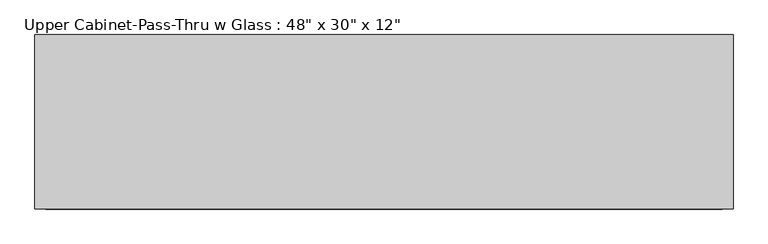
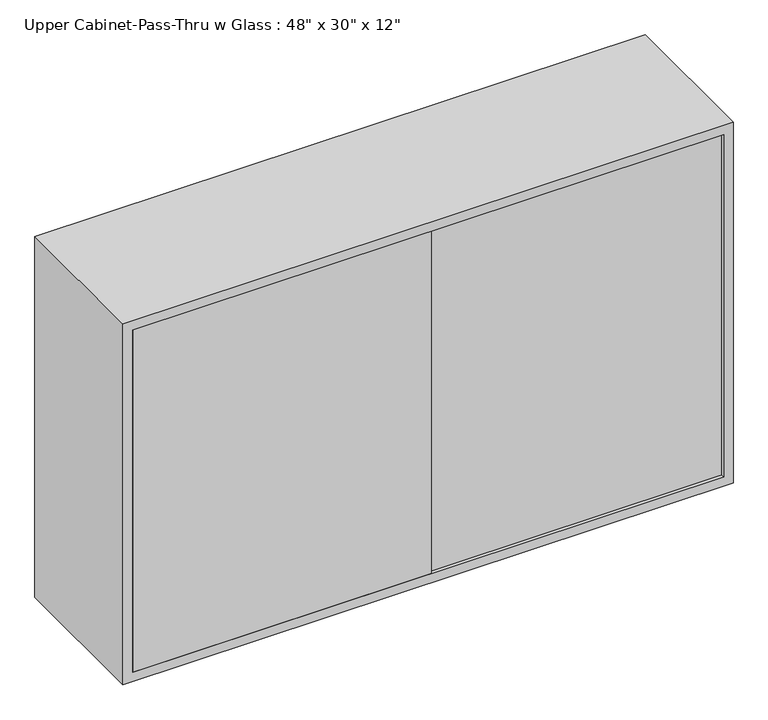
"""IFC4 building model written with IfcOpenShell, lengths in millimetres: furniture geometry."""

from ifc_helpers import new_model, si_unit, frame, origin, place, context, project, spatial, polyline, outline, extrude, source, transform, mapped, element, save


def furniture_f491f192(model_context):
    return source(origin(), model_context, "Body", "SweptSolid", [
        extrude(outline(polyline([(1371.6, 628.3377049), (2133.6, 628.3377049), (2133.6, -590.8622951), (1371.6, -590.8622951), (1371.6, 628.3377049)]), holes=[polyline([(1390.65, 609.2877049), (1390.65, -571.8122951), (2114.55, -571.8122951), (2114.55, 609.2877049), (1390.65, 609.2877049)])]), frame((0.0, -304.8, 0.0), z_axis=(0.0, 1.0, 0.0), x_axis=(0.0, 0.0, 1.0)), (0.0, 0.0, 1.0), 304.8),
        extrude(outline(polyline([(25.0877049, -304.8), (-571.8122951, -304.8), (-571.8122951, -298.45), (25.0877049, -298.45), (25.0877049, -304.8)])), frame((0.0, 0.0, 1390.65), z_axis=(0.0, 0.0, 1.0), x_axis=(1.0, 0.0, 0.0)), (0.0, 0.0, 1.0), 723.9),
        extrude(outline(polyline([(609.2877049, -6.35), (12.3877049, -6.35), (12.3877049, 0.0), (609.2877049, 0.0), (609.2877049, -6.35)])), frame((0.0, 0.0, 1390.65), z_axis=(0.0, 0.0, 1.0), x_axis=(1.0, 0.0, 0.0)), (0.0, 0.0, 1.0), 723.9),
        extrude(outline(polyline([(609.2877049, -298.45), (12.3877049, -298.45), (12.3877049, -292.1), (609.2877049, -292.1), (609.2877049, -298.45)])), frame((0.0, 0.0, 1390.65), z_axis=(0.0, 0.0, 1.0), x_axis=(1.0, 0.0, 0.0)), (0.0, 0.0, 1.0), 723.9),
        extrude(outline(polyline([(25.0877049, -12.7), (-571.8122951, -12.7), (-571.8122951, -6.35), (25.0877049, -6.35), (25.0877049, -12.7)])), frame((0.0, 0.0, 1390.65), z_axis=(0.0, 0.0, 1.0), x_axis=(1.0, 0.0, 0.0)), (0.0, 0.0, 1.0), 723.9),
        extrude(outline(polyline([(609.2877049, -285.75), (-571.8122951, -285.75), (-571.8122951, -19.05), (609.2877049, -19.05), (609.2877049, -285.75)])), frame((0.0, 0.0, 1873.25), z_axis=(0.0, 0.0, 1.0), x_axis=(1.0, 0.0, 0.0)), (0.0, 0.0, 1.0), 12.7),
        extrude(outline(polyline([(609.2877049, -285.75), (-571.8122951, -285.75), (-571.8122951, -19.05), (609.2877049, -19.05), (609.2877049, -285.75)])), frame((0.0, 0.0, 1619.25), z_axis=(0.0, 0.0, 1.0), x_axis=(1.0, 0.0, 0.0)), (0.0, 0.0, 1.0), 12.7),
    ])


if __name__ == "__main__":
    model = new_model("IFC4")
    model_context = context("Model", 3, world=origin())
    ifc_project = project(units=[si_unit("LENGTHUNIT", "METRE", prefix="MILLI")], contexts=[model_context])
    site = spatial("IfcSite", under=ifc_project)
    building = spatial("IfcBuilding", under=site)
    placement = place(None, origin())
    furniture_shape = furniture_f491f192(model_context)
    element("IfcFurniture", 1, ObjectType="Upper Cabinet-Pass-Thru w Glass : 48\" x 30\" x 12\"", at=placement, inside=building, context=model_context, shape_type="MappedRepresentation", body=[
        mapped(furniture_shape, transform((0.0, 0.0, 0.0), x_axis=(1.0, 0.0, 0.0), y_axis=(0.0, 1.0, 0.0), z_axis=(0.0, 0.0, 1.0))),
    ])
    save(model, "model.ifc")

# Revit data of these elements
# Type "Upper Cabinet-Pass-Thru w Glass : 48\" x 30\" x 12\""
#   Depth = 1 ft
#   Height = 2.5 ft
#   Top Of Cabinet = 7 ft
#   Width = 4 ft
#   Default Elevation = 0
# Element 1 (IfcFurniture, "Upper Cabinet-Pass-Thru w Glass : 48\" x 30\" x 12\"")
#   Materials on its faces: "Glass", "Cabinet"
# Materials
#   "Glass": class "Glass", colour RGB 0 128 192, transparency 0.75, Description = "Soda Lime Glass", Cost = 0
#   "Cabinet": colour RGB 204 122 2, transparency 0
